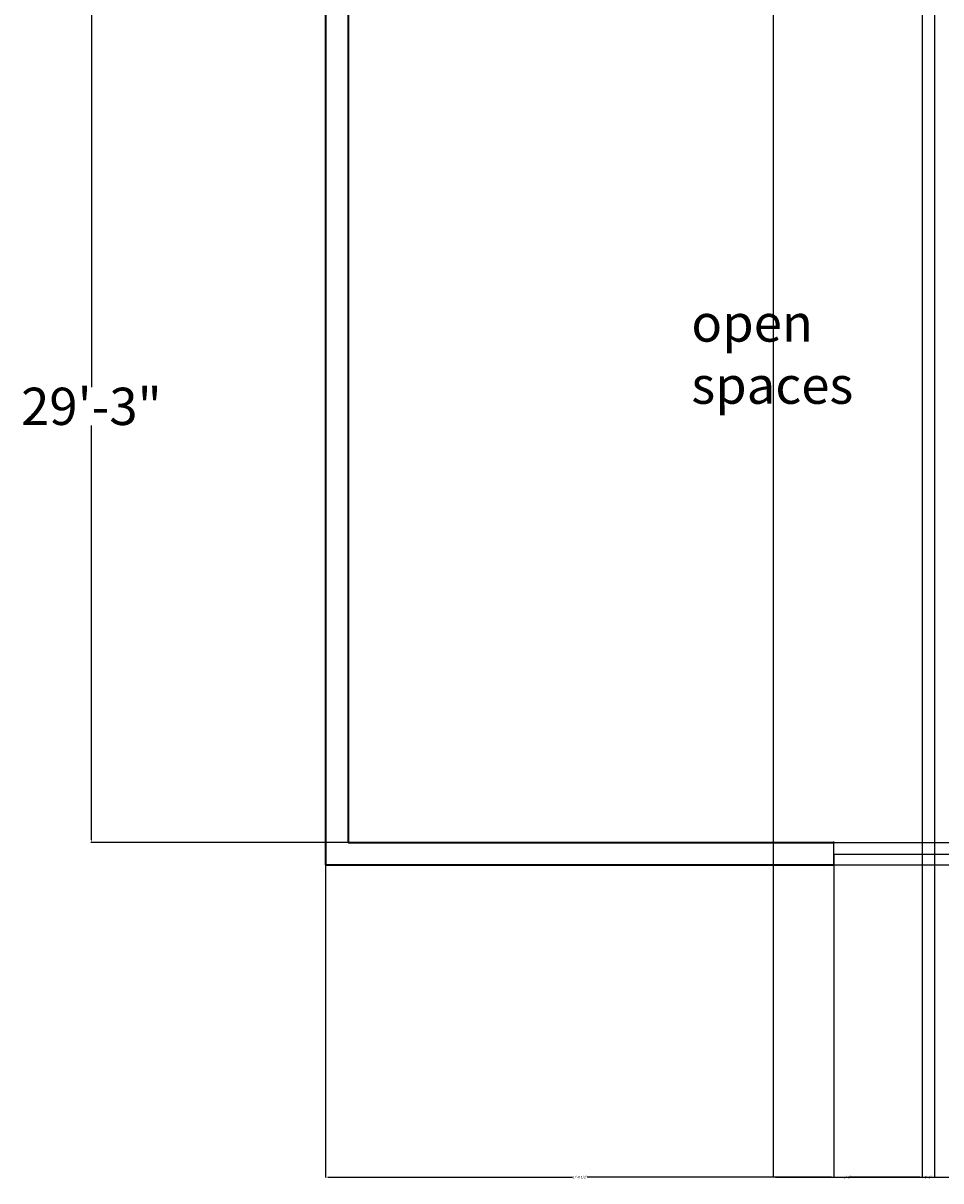
# Model space of a CAD drawing. Units: inches. Extents: x 371 to 1095, y -45 to 1219.
# Tile 1 of 18: x 371 to 740, y -45 to 421. Entities that reach past the tile are written whole.
import ezdxf

# ---------------------------------------------------------------- set-up
doc = ezdxf.new("R2010")
doc.units = ezdxf.units.IN
doc.header["$MEASUREMENT"] = 0
for name, color, linetype, lineweight in [('A-ANNO-DIMS', 2, 'Continuous', 18), ('A-AREA-IDEN', 7, 'Continuous', 18), ('A-WALL', 40, 'Continuous', 35), ('C-SITE-GATE', 3, 'Continuous', 25), ('C-SITE-WALL', 40, 'Continuous', 35)]:
    doc.layers.add(name, color=color, linetype=linetype, lineweight=lineweight)
doc.styles.get("Standard").update_dxf_attribs({"font": 'arial.ttf'})
doc.dimstyles.get("Standard").update_dxf_attribs({"dimtxt": 1, "dimasz": 1, "dimexe": 0.18, "dimexo": 0.0625, "dimgap": 0.09, "dimtad": 0, "dimtih": 1, "dimtoh": 1, "dimdec": 0, "dimzin": 0, "dimdsep": 46, "dimlunit": 3, "dimtxsty": 'Standard', "dimcen": 0.09, "dimadec": 0, "dimazin": 0, "dimtfac": 1, "dimtdec": 0, "dimtofl": 0, "dimtmove": 0, "dimatfit": 3, "dimfxl": 1, "dimtolj": 1, "dimtzin": 0, "dimarcsym": 0})

# ---------------------------------------------------------------- blocks, each defined once
blk = doc.blocks.new('*U18')
for p, q in [((-28, 0), (-28, -4)), ((0, 0), (0, -4))]:
    blk.add_line(p, q)
blk.add_lwpolyline([(0, 0), (-28, 0), (-28, -1.75), (0, -1.75)], close=True)
blk = doc.blocks.new('*D25')
at = {"layer": 'A-ANNO-DIMS', "color": 0, "lineweight": -2, "transparency": 16777216}
for p, q in [((501.75, 442.03), (398.38, 442.03)), ((398.56, 441.03), (398.56, 274.28)), ((398.56, 92.03), (398.56, 258.77)), ((501.75, 91.03), (398.38, 91.03))]:
    blk.add_line(p, q, dxfattribs=at)
at = {"layer": 'A-ANNO-DIMS', "color": 0, "transparency": 16777216}
for points in [[(398.4, 441.03), (398.73, 441.03), (398.56, 442.03)], [(398.4, 92.03), (398.73, 92.03), (398.56, 91.03)]]:
    blk.add_solid(points, dxfattribs=at)
at = {"layer": 'Defpoints', "color": 0, "transparency": 16777216}
for p in [(501.81, 442.03), (398.56, 91.03), (501.81, 91.03)]:
    blk.add_point(p, dxfattribs=at)
at = {"layer": 'A-ANNO-DIMS', "color": 0, "transparency": 16777216, "insert": (398.56, 266.53), "char_height": 1, "attachment_point": 5}
blk.add_mtext('\\A1;{\\H15x;29\'-3"}', dxfattribs=at)
blk = doc.blocks.new('*D52')
at = {"layer": 'A-ANNO-DIMS', "color": 0, "lineweight": -2, "transparency": 16777216}
for p, q in [((697.33, 81.96), (697.33, -43.83)), ((828.28, 81.96), (828.28, -43.83)), ((698.33, -43.65), (760.66, -43.65)), ((827.28, -43.65), (764.96, -43.65))]:
    blk.add_line(p, q, dxfattribs=at)
at = {"layer": 'A-ANNO-DIMS', "color": 0, "transparency": 16777216}
for points in [[(698.33, -43.48), (698.33, -43.82), (697.33, -43.65)], [(827.28, -43.48), (827.28, -43.82), (828.28, -43.65)]]:
    blk.add_solid(points, dxfattribs=at)
at = {"layer": 'Defpoints', "color": 0, "transparency": 16777216}
for p in [(697.33, 82.03), (828.28, 82.03), (828.28, -43.65)]:
    blk.add_point(p, dxfattribs=at)
at = {"layer": 'A-ANNO-DIMS', "color": 0, "transparency": 16777216, "insert": (762.81, -43.65), "char_height": 1, "attachment_point": 5}
blk.add_mtext('\\A1;10\'-11"', dxfattribs=at)
blk = doc.blocks.new('*D53')
at = {"layer": 'A-ANNO-DIMS', "color": 0, "lineweight": -2, "transparency": 16777216}
for p, q in [((492.81, 81.96), (492.81, -43.83)), ((697.33, 81.96), (697.33, -43.83)), ((493.81, -43.65), (592.15, -43.65)), ((696.33, -43.65), (598, -43.65))]:
    blk.add_line(p, q, dxfattribs=at)
at = {"layer": 'A-ANNO-DIMS', "color": 0, "transparency": 16777216}
for points in [[(493.81, -43.48), (493.81, -43.82), (492.81, -43.65)], [(696.33, -43.48), (696.33, -43.82), (697.33, -43.65)]]:
    blk.add_solid(points, dxfattribs=at)
at = {"layer": 'Defpoints', "color": 0, "transparency": 16777216}
for p in [(492.81, 82.03), (697.33, 82.03), (697.33, -43.65)]:
    blk.add_point(p, dxfattribs=at)
at = {"layer": 'A-ANNO-DIMS', "color": 0, "transparency": 16777216, "insert": (595.07, -43.65), "char_height": 1, "attachment_point": 5}
blk.add_mtext('\\A1;17\'-0 1/2"', dxfattribs=at)
blk = doc.blocks.new('*D54')
at = {"layer": 'A-ANNO-DIMS', "color": 0, "lineweight": -2, "transparency": 16777216}
for p, q in [((672.81, 924.96), (672.81, -43.83)), ((732.81, 924.96), (732.81, -43.83)), ((673.81, -43.65), (701.39, -43.65)), ((731.81, -43.65), (704.23, -43.65))]:
    blk.add_line(p, q, dxfattribs=at)
at = {"layer": 'A-ANNO-DIMS', "color": 0, "transparency": 16777216}
for points in [[(673.81, -43.48), (673.81, -43.82), (672.81, -43.65)], [(731.81, -43.48), (731.81, -43.82), (732.81, -43.65)]]:
    blk.add_solid(points, dxfattribs=at)
at = {"layer": 'Defpoints', "color": 0, "transparency": 16777216}
for p in [(672.81, 925.03), (732.81, 925.03), (732.81, -43.65)]:
    blk.add_point(p, dxfattribs=at)
at = {"layer": 'A-ANNO-DIMS', "color": 0, "transparency": 16777216, "insert": (702.81, -43.65), "char_height": 1, "attachment_point": 5}
blk.add_mtext('\\A1;5\'-0"', dxfattribs=at)
blk = doc.blocks.new('*D57')
at = {"layer": 'A-ANNO-DIMS', "color": 0, "lineweight": -2, "transparency": 16777216}
for p, q in [((732.81, 924.96), (732.81, -43.83)), ((737.81, 919.96), (737.81, -43.83)), ((731.81, -43.65), (730.81, -43.65)), ((738.81, -43.65), (739.81, -43.65))]:
    blk.add_line(p, q, dxfattribs=at)
at = {"layer": 'A-ANNO-DIMS', "color": 0, "transparency": 16777216}
for points in [[(731.81, -43.48), (731.81, -43.82), (732.81, -43.65)], [(738.81, -43.48), (738.81, -43.82), (737.81, -43.65)]]:
    blk.add_solid(points, dxfattribs=at)
at = {"layer": 'Defpoints', "color": 0, "transparency": 16777216}
for p in [(732.81, 925.03), (737.81, 920.03), (732.81, -43.65)]:
    blk.add_point(p, dxfattribs=at)
at = {"layer": 'A-ANNO-DIMS', "color": 0, "transparency": 16777216, "insert": (735.31, -43.65), "char_height": 1, "attachment_point": 5}
blk.add_mtext('\\A1;0\'-5"', dxfattribs=at)

msp = doc.modelspace()

# ---------------------------------------------------------------- linework, layer by layer
at = {"layer": 'A-WALL'}
msp.add_line((492.81, 982.03), (492.81, 82.03), dxfattribs=at)
at = {"layer": 'C-SITE-GATE'}
msp.add_line((697.33, 91.03), (828.28, 91.03), dxfattribs=at)
at = {"layer": 'C-SITE-WALL'}
for p, q in [((501.81, 442.03), (501.81, 91.03)), ((501.81, 91.03), (697.33, 91.03)), ((492.81, 82.03), (697.33, 82.03))]:
    msp.add_line(p, q, dxfattribs=at)

# ---------------------------------------------------------------- block references
at = {"layer": 'C-SITE-GATE', "xscale": 2.338360003491396, "yscale": 2.338360003491396, "zscale": 2.338360003491396, "rotation": 180}
msp.add_blockref('*U18', (697.33, 82.03), dxfattribs=at)

# ---------------------------------------------------------------- texts
at = {"layer": 'A-AREA-IDEN', "insert": (639.95, 307.56), "char_height": 15, "attachment_point": 1}
msp.add_mtext_dynamic_manual_height_columns('open spaces', width=103.7531, gutter_width=1, heights=[0], dxfattribs=at)

# ---------------------------------------------------------------- dimensions: what is measured, and where the dimension line sits
at = {"layer": 'A-ANNO-DIMS'}
for base, p1, p2, picture, middle in [((732.81, -43.65), (672.81, 925.03), (732.81, 925.03), '*D54', (702.81, -43.65)), ((732.81, -43.65), (737.81, 920.03), (732.81, 925.03), '*D57', (735.31, -43.65)), ((697.33, -43.65), (492.81, 82.03), (697.33, 82.03), '*D53', (595.07, -43.65)), ((828.282, -43.649), (697.3338, 82.0251), (828.282, 82.0251), '*D52', (762.8079, -43.649))]:
    dim = msp.add_linear_dim(base=base, p1=p1, p2=p2, dimstyle='Standard', override={"dimdec": 1, "dimlfac": 1, "dimrnd": 0, "dimzin": 1, "dimdsep": 46, "dimlunit": 4, "dimfrac": 2}, dxfattribs=at)
    dim.commit()
    dim.dimension.update_dxf_attribs({"geometry": picture, "text_midpoint": middle})
dim = msp.add_linear_dim(base=(398.56, 91.03), p1=(501.81, 442.03), p2=(501.81, 91.03), angle=90, text='{\\H15x;<>}', dimstyle='Standard', override={"dimclrd": 0, "dimclre": 0, "dimclrt": 0}, dxfattribs=at)
dim.commit()
dim.dimension.update_dxf_attribs({"geometry": '*D25', "text_midpoint": (398.56, 266.53)})

doc.saveas('drawing.dxf')
